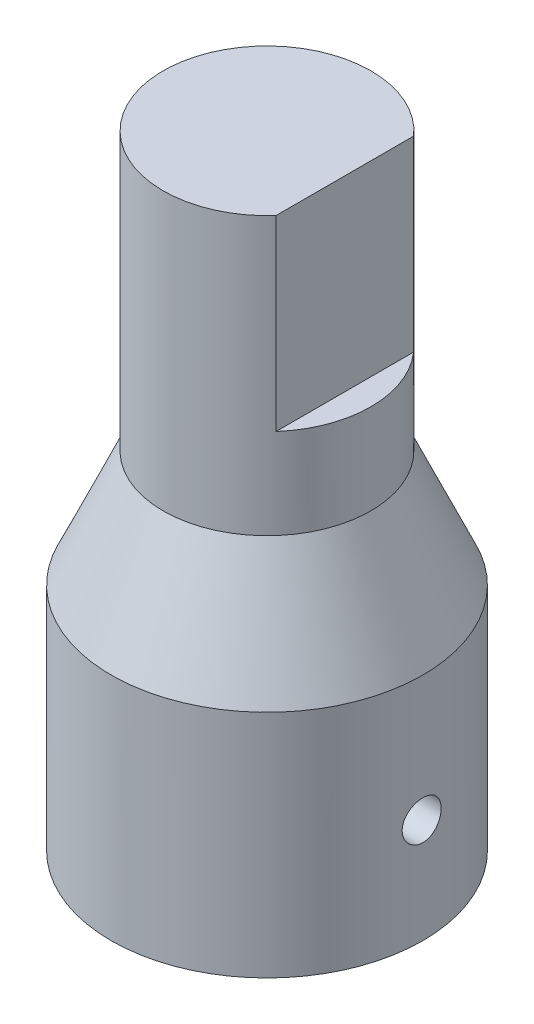
SolidWorks part; units mm, degrees
material "Plain Carbon Steel"
ref_plane "Front Plane" through (0, 0, 0) normal (0, 0, 1) x (1, 0, 0)
ref_plane "Top Plane" through (0, 0, 0) normal (0, 1, 0) x (1, 0, 0)
ref_plane "Right Plane" through (0, 0, 0) normal (1, 0, 0) x (0, 0, -1)
sketch "Base Cylinder Sketch Ø19.05" plane through (0, 0, 0) normal (0, 1, 0) x (1, 0, 0)
  circle A0 centre (0, 0) radius 9.525
  dimension "D1" = 19.05
extrude "Base Cylinder Ø19.05" add sketch "Base Cylinder Sketch Ø19.05" along normal blind 14.06
ref_plane "Taper Top Plane" through (0, 21.16, 0) normal (0, 1, 0) x (1, 0, 0)
sketch "Taper Top Sketch Ø12.7" plane through (0, 21.16, 0) normal (0, 1, 0) x (1, 0, 0)
  circle A0 centre (0, 0) radius 6.35
  dimension "D1" = 12.7
loft "Taper Loft" add profiles "Taper Top Sketch Ø12.7" section "Taper Top Sketch Ø12.7" section edge at (0, 14.06, 9.525)
sketch "Shank Sketch" plane through (0, 21.16, 0) normal (0, 1, 0) x (1, 0, 0)
  circle A1 centre (0, 0) radius 6.35
  circle A2 centre (0, 0) radius 6.35
  dimension "D1" = 0
extrude "Shank Ø12.7" add sketch "Shank Sketch" along normal blind 16.94
sketch "Shank Flat Sketch" plane through (0, 0, 0) normal (0, 0, 1) x (1, 0, 0)
  line L1 (6.35, 38.1) -> (4.76, 38.1)
  line L2 (6.35, 38.1) -> (6.35, 26.67)
  line L3 (6.35, 26.67) -> (4.76, 26.67)
  line L4 (4.76, 38.1) -> (4.76, 26.67)
  dimension "D1" = 11.43
  dimension "D2" = 11.11
extrude "Shank Flat" cut sketch "Shank Flat Sketch" against normal mid plane 16.94
sketch "Bore Sketch Ø11.11" plane through (0, 0, 0) normal (0, -1, 0) x (1, 0, 0)
  circle A0 centre (0, 0) radius 6.35
  dimension "D1" = 12.7
extrude "Bore Ø11.11" cut sketch "Bore Sketch Ø11.11" against normal blind 14.06
sketch "Cross Hole Sketch Ø2.38" plane through (0, 0, 0) normal (1, 0, 0) x (0, 0, -1)
  circle A0 centre (0, 6.38) radius 1.19
  dimension "D2" = 2.38
  dimension "D1" = 6.38
extrude "Cross Hole Ø2.38" cut sketch "Cross Hole Sketch Ø2.38" along normal blind 14.06
